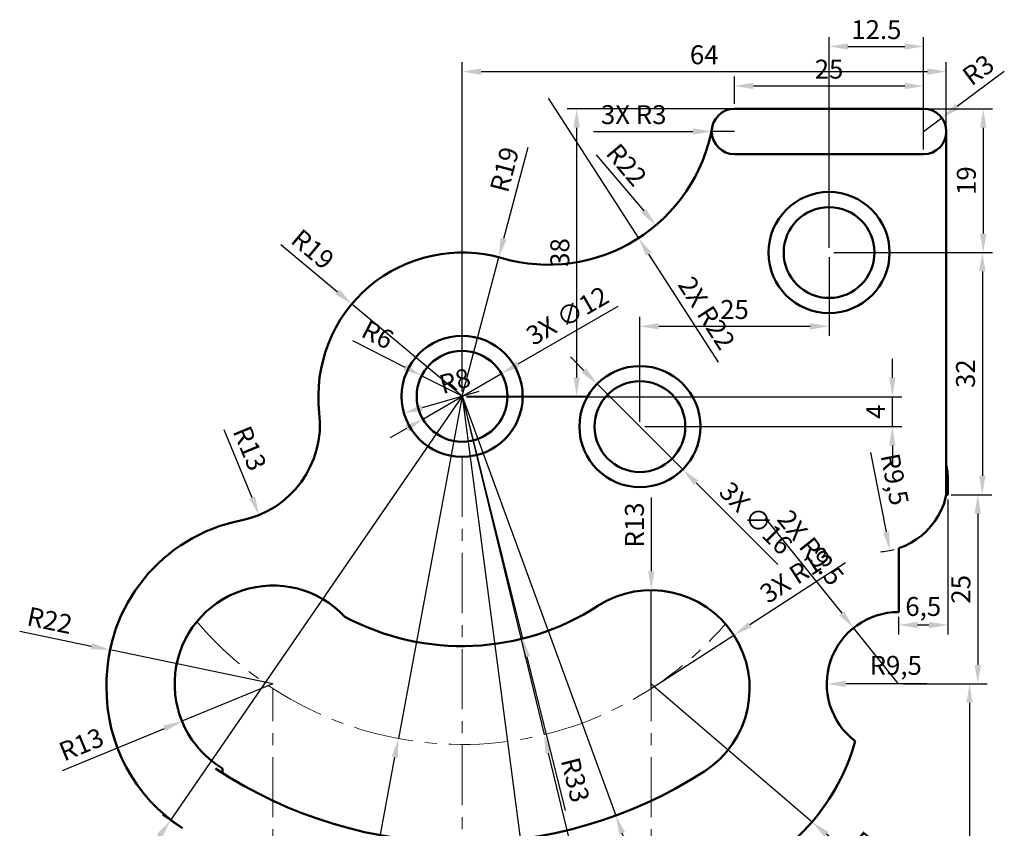
# Model space of a CAD drawing. Units: millimetres. Extents: x 2366 to 2507, y 1526 to 1734.
# Tile 2 of 2: x 2377 to 2507, y 1627 to 1734. Entities that reach past the tile are written whole.
import ezdxf

# ---------------------------------------------------------------- set-up
doc = ezdxf.new("R2010")
doc.units = ezdxf.units.MM
doc.linetypes.add('CENTER', pattern=[50.8, 31.75, -6.35, 6.35, -6.35])
for name, color, linetype, lineweight in [('M-CNTR', 4, 'CENTER', 18), ('M-DIMS', 2, 'Continuous', 25), ('M-OUTL', 7, 'Continuous', 50)]:
    doc.layers.add(name, color=color, linetype=linetype, lineweight=lineweight)
doc.styles.get("Standard").update_dxf_attribs({"font": 'arial.ttf'})
doc.dimstyles.new('ISO-25', dxfattribs={"dimtxt": 2.5, "dimasz": 2.5, "dimexe": 1.25, "dimexo": 0.625, "dimtad": 1, "dimtxsty": 'Standard', "dimcen": 2.5, "dimadec": 0, "dimazin": 0, "dimtfac": 1, "dimtmove": 0, "dimatfit": 3, "dimfxl": 1, "dimarcsym": 0})

# ---------------------------------------------------------------- blocks, each defined once
blk = doc.blocks.new('*D1')
at = {"layer": 'Defpoints', "color": 0, "transparency": 16777216}
for p in [(2496.16, 1724.79), (2471.16, 1721.78), (2496.16, 1721.78)]:
    blk.add_point(p, dxfattribs=at)
at = {"layer": 'M-DIMS', "color": 0, "lineweight": -2, "transparency": 16777216}
for p, q in [((2471.16, 1722.41), (2471.16, 1726.04)), ((2496.16, 1722.41), (2496.16, 1726.04)), ((2473.66, 1724.79), (2493.66, 1724.79))]:
    blk.add_line(p, q, dxfattribs=at)
at = {"layer": 'M-DIMS', "color": 0, "transparency": 16777216}
for points in [[(2473.66, 1725.21), (2473.66, 1724.37), (2471.16, 1724.79)], [(2493.66, 1725.21), (2493.66, 1724.37), (2496.16, 1724.79)]]:
    blk.add_solid(points, dxfattribs=at)
at = {"layer": 'M-DIMS', "color": 0, "transparency": 16777216, "insert": (2483.66, 1726.69), "char_height": 2.5, "attachment_point": 5}
blk.add_mtext('25', dxfattribs=at)
blk = doc.blocks.new('*D2')
at = {"layer": 'Defpoints', "color": 0, "transparency": 16777216}
for p in [(2499.16, 1726.69), (2499.16, 1718.78), (2435.16, 1683.78)]:
    blk.add_point(p, dxfattribs=at)
at = {"layer": 'M-DIMS', "color": 0, "lineweight": -2, "transparency": 16777216}
for p, q in [((2435.16, 1684.41), (2435.16, 1727.94)), ((2499.16, 1719.41), (2499.16, 1727.94)), ((2437.66, 1726.69), (2496.66, 1726.69))]:
    blk.add_line(p, q, dxfattribs=at)
at = {"layer": 'M-DIMS', "color": 0, "transparency": 16777216}
for points in [[(2437.66, 1727.11), (2437.66, 1726.27), (2435.16, 1726.69)], [(2496.66, 1727.11), (2496.66, 1726.27), (2499.16, 1726.69)]]:
    blk.add_solid(points, dxfattribs=at)
at = {"layer": 'M-DIMS', "color": 0, "transparency": 16777216, "insert": (2467.16, 1728.59), "char_height": 2.5, "attachment_point": 5}
blk.add_mtext('64', dxfattribs=at)
blk = doc.blocks.new('*D3')
at = {"layer": 'Defpoints', "color": 0, "transparency": 16777216}
for p in [(2471.16, 1721.78), (2435.16, 1683.78), (2450.3, 1683.78)]:
    blk.add_point(p, dxfattribs=at)
at = {"layer": 'M-DIMS', "color": 0, "lineweight": -2, "transparency": 16777216}
for p, q in [((2470.54, 1721.78), (2449.05, 1721.78)), ((2450.3, 1719.28), (2450.3, 1686.28)), ((2435.79, 1683.78), (2451.55, 1683.78))]:
    blk.add_line(p, q, dxfattribs=at)
at = {"layer": 'M-DIMS', "color": 0, "transparency": 16777216}
for points in [[(2449.89, 1719.28), (2450.72, 1719.28), (2450.3, 1721.78)], [(2449.89, 1686.28), (2450.72, 1686.28), (2450.3, 1683.78)]]:
    blk.add_solid(points, dxfattribs=at)
at = {"layer": 'M-DIMS', "color": 0, "transparency": 16777216, "insert": (2448.4, 1702.78), "char_height": 2.5, "attachment_point": 5, "rotation": 90}
blk.add_mtext('38', dxfattribs=at)
blk = doc.blocks.new('*D4')
at = {"layer": 'Defpoints', "color": 0, "transparency": 16777216}
for p in [(2483.66, 1702.78), (2483.66, 1693.03), (2458.66, 1679.78)]:
    blk.add_point(p, dxfattribs=at)
at = {"layer": 'M-DIMS', "color": 0, "lineweight": -2, "transparency": 16777216}
for p, q in [((2483.66, 1702.16), (2483.66, 1691.78)), ((2458.66, 1680.41), (2458.66, 1694.28)), ((2461.16, 1693.03), (2481.16, 1693.03))]:
    blk.add_line(p, q, dxfattribs=at)
at = {"layer": 'M-DIMS', "color": 0, "transparency": 16777216}
for points in [[(2461.16, 1693.45), (2461.16, 1692.62), (2458.66, 1693.03)], [(2481.16, 1693.45), (2481.16, 1692.62), (2483.66, 1693.03)]]:
    blk.add_solid(points, dxfattribs=at)
at = {"layer": 'M-DIMS', "color": 0, "transparency": 16777216, "insert": (2471.16, 1694.93), "char_height": 2.5, "attachment_point": 5}
blk.add_mtext('25', dxfattribs=at)
blk = doc.blocks.new('*D5')
at = {"layer": 'Defpoints', "color": 0, "transparency": 16777216}
for p in [(2496.16, 1721.78), (2483.66, 1702.78), (2504.03, 1702.78)]:
    blk.add_point(p, dxfattribs=at)
at = {"layer": 'M-DIMS', "color": 0, "lineweight": -2, "transparency": 16777216}
for p, q in [((2496.79, 1721.78), (2505.28, 1721.78)), ((2504.03, 1719.28), (2504.03, 1705.28)), ((2484.29, 1702.78), (2505.28, 1702.78))]:
    blk.add_line(p, q, dxfattribs=at)
at = {"layer": 'M-DIMS', "color": 0, "transparency": 16777216}
for points in [[(2503.62, 1719.28), (2504.45, 1719.28), (2504.03, 1721.78)], [(2503.62, 1705.28), (2504.45, 1705.28), (2504.03, 1702.78)]]:
    blk.add_solid(points, dxfattribs=at)
at = {"layer": 'M-DIMS', "color": 0, "transparency": 16777216, "insert": (2502.13, 1712.28), "char_height": 2.5, "attachment_point": 5, "rotation": 90}
blk.add_mtext('19', dxfattribs=at)
blk = doc.blocks.new('*D6')
at = {"layer": 'Defpoints', "color": 0, "transparency": 16777216}
for p in [(2483.66, 1702.78), (2499.36, 1670.78), (2503.92, 1670.78)]:
    blk.add_point(p, dxfattribs=at)
at = {"layer": 'M-DIMS', "color": 0, "lineweight": -2, "transparency": 16777216}
for p, q in [((2484.29, 1702.78), (2505.17, 1702.78)), ((2503.92, 1700.28), (2503.92, 1673.28)), ((2499.99, 1670.78), (2505.17, 1670.78))]:
    blk.add_line(p, q, dxfattribs=at)
at = {"layer": 'M-DIMS', "color": 0, "transparency": 16777216}
for points in [[(2503.5, 1700.28), (2504.34, 1700.28), (2503.92, 1702.78)], [(2503.5, 1673.28), (2504.34, 1673.28), (2503.92, 1670.78)]]:
    blk.add_solid(points, dxfattribs=at)
at = {"layer": 'M-DIMS', "color": 0, "transparency": 16777216, "insert": (2502.02, 1686.78), "char_height": 2.5, "attachment_point": 5, "rotation": 90}
blk.add_mtext('32', dxfattribs=at)
blk = doc.blocks.new('*D7')
at = {"layer": 'Defpoints', "color": 0, "transparency": 16777216}
for p in [(2499.16, 1670.78), (2492.86, 1645.78), (2503.32, 1645.78)]:
    blk.add_point(p, dxfattribs=at)
at = {"layer": 'M-DIMS', "color": 0, "lineweight": -2, "transparency": 16777216}
for p, q in [((2499.79, 1670.78), (2504.57, 1670.78)), ((2503.32, 1668.28), (2503.32, 1648.28)), ((2493.49, 1645.78), (2504.57, 1645.78))]:
    blk.add_line(p, q, dxfattribs=at)
at = {"layer": 'M-DIMS', "color": 0, "transparency": 16777216}
for points in [[(2502.9, 1668.28), (2503.73, 1668.28), (2503.32, 1670.78)], [(2502.9, 1648.28), (2503.73, 1648.28), (2503.32, 1645.78)]]:
    blk.add_solid(points, dxfattribs=at)
at = {"layer": 'M-DIMS', "color": 0, "transparency": 16777216, "insert": (2501.41, 1658.28), "char_height": 2.5, "attachment_point": 5, "rotation": 90}
blk.add_mtext('25', dxfattribs=at)
blk = doc.blocks.new('*D8')
at = {"layer": 'Defpoints', "color": 0, "transparency": 16777216}
for p in [(2492.86, 1645.78), (2488.16, 1594.78), (2502.23, 1594.78)]:
    blk.add_point(p, dxfattribs=at)
at = {"layer": 'M-DIMS', "color": 0, "lineweight": -2, "transparency": 16777216}
for p, q in [((2493.49, 1645.78), (2503.48, 1645.78)), ((2502.23, 1643.28), (2502.23, 1597.28)), ((2488.79, 1594.78), (2503.48, 1594.78))]:
    blk.add_line(p, q, dxfattribs=at)
at = {"layer": 'M-DIMS', "color": 0, "transparency": 16777216}
for points in [[(2501.81, 1643.28), (2502.64, 1643.28), (2502.23, 1645.78)], [(2501.81, 1597.28), (2502.64, 1597.28), (2502.23, 1594.78)]]:
    blk.add_solid(points, dxfattribs=at)
at = {"layer": 'M-DIMS', "color": 0, "transparency": 16777216, "insert": (2500.33, 1620.28), "char_height": 2.5, "attachment_point": 5, "rotation": 90}
blk.add_mtext('51', dxfattribs=at)
blk = doc.blocks.new('*D9')
at = {"layer": 'Defpoints', "color": 0, "transparency": 16777216}
for p in [(2499.36, 1670.78), (2492.86, 1655.28), (2499.36, 1653.57)]:
    blk.add_point(p, dxfattribs=at)
at = {"layer": 'M-DIMS', "color": 0, "lineweight": -2, "transparency": 16777216}
for p, q in [((2499.36, 1670.16), (2499.36, 1652.32)), ((2492.86, 1654.66), (2492.86, 1652.32)), ((2495.36, 1653.57), (2496.86, 1653.57))]:
    blk.add_line(p, q, dxfattribs=at)
at = {"layer": 'M-DIMS', "color": 0, "transparency": 16777216}
for points in [[(2495.36, 1653.98), (2495.36, 1653.15), (2492.86, 1653.57)], [(2496.86, 1653.98), (2496.86, 1653.15), (2499.36, 1653.57)]]:
    blk.add_solid(points, dxfattribs=at)
at = {"layer": 'M-DIMS', "color": 0, "transparency": 16777216, "insert": (2496.11, 1655.69), "char_height": 2.5, "attachment_point": 5}
blk.add_mtext('6,5', dxfattribs=at)
blk = doc.blocks.new('*D18')
at = {"layer": 'Defpoints', "color": 0, "transparency": 16777216}
for p in [(2435.16, 1683.78), (2426.73, 1638.56)]:
    blk.add_point(p, dxfattribs=at)
at = {"layer": 'M-DIMS', "color": 0, "lineweight": -2, "transparency": 16777216}
for p, q in [((2435.16, 1683.78), (2426.73, 1638.56)), ((2422.8, 1617.49), (2426.27, 1636.1))]:
    blk.add_line(p, q, dxfattribs=at)
at = {"layer": 'M-DIMS', "color": 0, "transparency": 16777216}
blk.add_solid([(2425.86, 1636.18), (2426.68, 1636.03), (2426.73, 1638.56)], dxfattribs=at)
at = {"layer": 'M-DIMS', "color": 0, "transparency": 16777216, "insert": (2421.6, 1621.39), "char_height": 2.5, "attachment_point": 5, "rotation": 79.4409}
blk.add_mtext('R46', dxfattribs=at)
blk = doc.blocks.new('*D19')
at = {"layer": 'Defpoints', "color": 0, "transparency": 16777216}
for p in [(2435.16, 1683.78), (2396.6, 1627.77)]:
    blk.add_point(p, dxfattribs=at)
at = {"layer": 'M-DIMS', "color": 0, "lineweight": -2, "transparency": 16777216}
for p, q in [((2435.16, 1683.78), (2396.6, 1627.77)), ((2389.67, 1617.7), (2395.18, 1625.71))]:
    blk.add_line(p, q, dxfattribs=at)
blk.add_arc((2435.16, 1683.78), 68, 234.401, 236.5526, dxfattribs=at)
at = {"layer": 'M-DIMS', "color": 0, "transparency": 16777216}
blk.add_solid([(2394.84, 1625.95), (2395.53, 1625.48), (2396.6, 1627.77)], dxfattribs=at)
at = {"layer": 'M-DIMS', "color": 0, "transparency": 16777216, "insert": (2390.15, 1621.75), "char_height": 2.5, "attachment_point": 5, "rotation": 55.4543}
blk.add_mtext('R68', dxfattribs=at)
blk = doc.blocks.new('*D20')
at = {"layer": 'Defpoints', "color": 0, "transparency": 16777216}
for p in [(2388.62, 1650.27), (2410.16, 1645.78)]:
    blk.add_point(p, dxfattribs=at)
at = {"layer": 'M-DIMS', "color": 0, "lineweight": -2, "transparency": 16777216}
for p, q in [((2376.68, 1652.75), (2386.18, 1650.78)), ((2410.16, 1645.78), (2388.62, 1650.27))]:
    blk.add_line(p, q, dxfattribs=at)
at = {"layer": 'M-DIMS', "color": 0, "transparency": 16777216}
blk.add_solid([(2386.26, 1651.18), (2386.09, 1650.37), (2388.62, 1650.27)], dxfattribs=at)
at = {"layer": 'M-DIMS', "color": 0, "transparency": 16777216, "insert": (2380.59, 1653.86), "char_height": 2.5, "attachment_point": 5, "rotation": 348.2349}
blk.add_mtext('R22', dxfattribs=at)
blk = doc.blocks.new('*D21')
at = {"layer": 'Defpoints', "color": 0, "transparency": 16777216}
for p in [(2410.16, 1645.78), (2398.13, 1640.85)]:
    blk.add_point(p, dxfattribs=at)
at = {"layer": 'M-DIMS', "color": 0, "lineweight": -2, "transparency": 16777216}
for p, q in [((2410.16, 1645.78), (2398.13, 1640.85)), ((2382.33, 1634.36), (2395.82, 1639.9))]:
    blk.add_line(p, q, dxfattribs=at)
at = {"layer": 'M-DIMS', "color": 0, "transparency": 16777216}
blk.add_solid([(2395.66, 1640.28), (2395.98, 1639.51), (2398.13, 1640.85)], dxfattribs=at)
at = {"layer": 'M-DIMS', "color": 0, "transparency": 16777216, "insert": (2384.95, 1637.49), "char_height": 2.5, "attachment_point": 5, "rotation": 22.313}
blk.add_mtext('R13', dxfattribs=at)
blk = doc.blocks.new('*D22')
at = {"layer": 'Defpoints', "color": 0, "transparency": 16777216}
for p in [(2403.37, 1680.12), (2408.33, 1668.1)]:
    blk.add_point(p, dxfattribs=at)
at = {"layer": 'M-DIMS', "color": 0, "lineweight": -2, "transparency": 16777216}
blk.add_line((2403.67, 1679.4), (2407.38, 1670.41), dxfattribs=at)
at = {"layer": 'M-DIMS', "color": 0, "transparency": 16777216}
blk.add_solid([(2407.77, 1670.57), (2407, 1670.25), (2408.33, 1668.1)], dxfattribs=at)
at = {"layer": 'M-DIMS', "color": 0, "transparency": 16777216, "insert": (2406.81, 1676.79), "char_height": 2.5, "attachment_point": 5, "rotation": 292.4423}
blk.add_mtext('R13', dxfattribs=at)
blk = doc.blocks.new('*D24')
at = {"layer": 'Defpoints', "color": 0, "transparency": 16777216}
for p in [(2460.16, 1645.78), (2481.41, 1627.54)]:
    blk.add_point(p, dxfattribs=at)
at = {"layer": 'M-DIMS', "color": 0, "lineweight": -2, "transparency": 16777216}
for p, q in [((2460.16, 1645.78), (2481.41, 1627.54)), ((2490.69, 1619.58), (2483.3, 1625.92))]:
    blk.add_line(p, q, dxfattribs=at)
at = {"layer": 'M-DIMS', "color": 0, "transparency": 16777216}
blk.add_solid([(2483.58, 1626.23), (2483.03, 1625.6), (2481.41, 1627.54)], dxfattribs=at)
at = {"layer": 'M-DIMS', "color": 0, "transparency": 16777216, "insert": (2489.18, 1623.38), "char_height": 2.5, "attachment_point": 5, "rotation": 319.3585}
blk.add_mtext('R28', dxfattribs=at)
blk = doc.blocks.new('*D25')
at = {"layer": 'Defpoints', "color": 0, "transparency": 16777216}
for p in [(2483.36, 1645.78), (2492.86, 1645.78)]:
    blk.add_point(p, dxfattribs=at)
at = {"layer": 'M-DIMS', "color": 0, "lineweight": -2, "transparency": 16777216}
blk.add_line((2496.58, 1645.78), (2485.86, 1645.78), dxfattribs=at)
at = {"layer": 'M-DIMS', "color": 0, "transparency": 16777216}
blk.add_solid([(2485.86, 1646.2), (2485.86, 1645.36), (2483.36, 1645.78)], dxfattribs=at)
at = {"layer": 'M-DIMS', "color": 0, "transparency": 16777216, "insert": (2492.47, 1647.91), "char_height": 2.5, "attachment_point": 5}
blk.add_mtext('R9,5', dxfattribs=at)
blk = doc.blocks.new('*D26')
at = {"layer": 'Defpoints', "color": 0, "transparency": 16777216}
for p in [(2489.86, 1672.73), (2491.7, 1663.41)]:
    blk.add_point(p, dxfattribs=at)
at = {"layer": 'M-DIMS', "color": 0, "lineweight": -2, "transparency": 16777216}
blk.add_line((2489.15, 1676.37), (2491.21, 1665.86), dxfattribs=at)
blk.add_arc((2489.86, 1672.73), 9.5, 273.5778, 284.639, dxfattribs=at)
at = {"layer": 'M-DIMS', "color": 0, "transparency": 16777216}
blk.add_solid([(2491.62, 1665.94), (2490.8, 1665.78), (2491.7, 1663.41)], dxfattribs=at)
at = {"layer": 'M-DIMS', "color": 0, "transparency": 16777216, "insert": (2492.03, 1672.75), "char_height": 2.5, "attachment_point": 5, "rotation": 281.1167}
blk.add_mtext('R9,5', dxfattribs=at)
blk = doc.blocks.new('*D27')
at = {"layer": 'Defpoints', "color": 0, "transparency": 16777216}
for p in [(2460.16, 1658.17), (2460.16, 1645.17)]:
    blk.add_point(p, dxfattribs=at)
at = {"layer": 'M-DIMS', "color": 0, "lineweight": -2, "transparency": 16777216}
for p, q in [((2460.16, 1670.39), (2460.16, 1660.67)), ((2460.16, 1645.17), (2460.16, 1658.17))]:
    blk.add_line(p, q, dxfattribs=at)
at = {"layer": 'M-DIMS', "color": 0, "transparency": 16777216}
blk.add_solid([(2459.74, 1660.67), (2460.58, 1660.67), (2460.16, 1658.17)], dxfattribs=at)
at = {"layer": 'M-DIMS', "color": 0, "transparency": 16777216, "insert": (2458.26, 1666.78), "char_height": 2.5, "attachment_point": 5, "rotation": 90}
blk.add_mtext('R13', dxfattribs=at)
blk = doc.blocks.new('*D28')
at = {"layer": 'Defpoints', "color": 0, "transparency": 16777216}
for p in [(2435.16, 1683.78), (2427.47, 1681.57)]:
    blk.add_point(p, dxfattribs=at)
at = {"layer": 'M-DIMS', "color": 0, "lineweight": -2, "transparency": 16777216}
blk.add_line((2437.36, 1684.41), (2429.88, 1682.26), dxfattribs=at)
at = {"layer": 'M-DIMS', "color": 0, "transparency": 16777216}
blk.add_solid([(2429.76, 1682.66), (2429.99, 1681.86), (2427.47, 1681.57)], dxfattribs=at)
at = {"layer": 'M-DIMS', "color": 0, "transparency": 16777216, "insert": (2434.29, 1685.51), "char_height": 2.5, "attachment_point": 5, "rotation": 16.0232}
blk.add_mtext('R8', dxfattribs=at)
blk = doc.blocks.new('*D29')
at = {"layer": 'Defpoints', "color": 0, "transparency": 16777216}
for p in [(2429.81, 1686.5), (2435.16, 1683.78)]:
    blk.add_point(p, dxfattribs=at)
at = {"layer": 'M-DIMS', "color": 0, "lineweight": -2, "transparency": 16777216}
for p, q in [((2420.65, 1691.15), (2427.58, 1687.63)), ((2435.16, 1683.78), (2429.81, 1686.5))]:
    blk.add_line(p, q, dxfattribs=at)
at = {"layer": 'M-DIMS', "color": 0, "transparency": 16777216}
blk.add_solid([(2427.77, 1688), (2427.39, 1687.26), (2429.81, 1686.5)], dxfattribs=at)
at = {"layer": 'M-DIMS', "color": 0, "transparency": 16777216, "insert": (2423.86, 1691.65), "char_height": 2.5, "attachment_point": 5, "rotation": 333.0794}
blk.add_mtext('R6', dxfattribs=at)
blk = doc.blocks.new('*D30')
at = {"layer": 'Defpoints', "color": 0, "transparency": 16777216}
for p in [(2420.6, 1695.98), (2435.16, 1683.78)]:
    blk.add_point(p, dxfattribs=at)
at = {"layer": 'M-DIMS', "color": 0, "lineweight": -2, "transparency": 16777216}
for p, q in [((2411.22, 1703.84), (2418.68, 1697.59)), ((2435.16, 1683.78), (2420.6, 1695.98))]:
    blk.add_line(p, q, dxfattribs=at)
at = {"layer": 'M-DIMS', "color": 0, "transparency": 16777216}
blk.add_solid([(2418.95, 1697.91), (2418.41, 1697.27), (2420.6, 1695.98)], dxfattribs=at)
at = {"layer": 'M-DIMS', "color": 0, "transparency": 16777216, "insert": (2415.21, 1702.97), "char_height": 2.5, "attachment_point": 5, "rotation": 320.0449}
blk.add_mtext('R19', dxfattribs=at)
blk = doc.blocks.new('*D31')
at = {"layer": 'Defpoints', "color": 0, "transparency": 16777216}
for p in [(2446.55, 1723.17), (2460.77, 1706.38)]:
    blk.add_point(p, dxfattribs=at)
at = {"layer": 'M-DIMS', "color": 0, "lineweight": -2, "transparency": 16777216}
blk.add_line((2452.89, 1715.69), (2459.16, 1708.29), dxfattribs=at)
at = {"layer": 'M-DIMS', "color": 0, "transparency": 16777216}
blk.add_solid([(2459.47, 1708.56), (2458.84, 1708.02), (2460.77, 1706.38)], dxfattribs=at)
at = {"layer": 'M-DIMS', "color": 0, "transparency": 16777216, "insert": (2456.65, 1714.16), "char_height": 2.5, "attachment_point": 5, "rotation": 310.2815}
blk.add_mtext('R22', dxfattribs=at)
blk = doc.blocks.new('*D32')
at = {"layer": 'Defpoints', "color": 0, "transparency": 16777216}
for p in [(2498.57, 1720.57), (2496.16, 1718.78)]:
    blk.add_point(p, dxfattribs=at)
at = {"layer": 'M-DIMS', "color": 0, "lineweight": -2, "transparency": 16777216}
for p, q in [((2506.82, 1726.7), (2500.58, 1722.06)), ((2496.16, 1718.78), (2498.57, 1720.57))]:
    blk.add_line(p, q, dxfattribs=at)
at = {"layer": 'M-DIMS', "color": 0, "transparency": 16777216}
blk.add_solid([(2500.33, 1722.39), (2500.83, 1721.73), (2498.57, 1720.57)], dxfattribs=at)
at = {"layer": 'M-DIMS', "color": 0, "transparency": 16777216, "insert": (2503.57, 1726.65), "char_height": 2.5, "attachment_point": 5, "rotation": 36.6003}
blk.add_mtext('R3', dxfattribs=at)
blk = doc.blocks.new('*D33')
at = {"layer": 'Defpoints', "color": 0, "transparency": 16777216}
for p in [(2435.12, 1683.73), (2492.03, 1683.73), (2458.66, 1679.78)]:
    blk.add_point(p, dxfattribs=at)
at = {"layer": 'M-DIMS', "color": 0, "lineweight": -2, "transparency": 16777216}
for p, q in [((2492.03, 1686.23), (2492.03, 1688.73)), ((2435.75, 1683.73), (2493.28, 1683.73)), ((2492.03, 1679.78), (2492.03, 1683.73)), ((2459.29, 1679.78), (2493.28, 1679.78)), ((2492.03, 1677.28), (2492.03, 1674.78))]:
    blk.add_line(p, q, dxfattribs=at)
at = {"layer": 'M-DIMS', "color": 0, "transparency": 16777216}
for points in [[(2491.61, 1686.23), (2492.44, 1686.23), (2492.03, 1683.73)], [(2491.61, 1677.28), (2492.44, 1677.28), (2492.03, 1679.78)]]:
    blk.add_solid(points, dxfattribs=at)
at = {"layer": 'M-DIMS', "color": 0, "transparency": 16777216, "insert": (2490.15, 1681.75), "char_height": 2.5, "attachment_point": 5, "rotation": 90}
blk.add_mtext('4', dxfattribs=at)
blk = doc.blocks.new('MOUNT-HOLE-D12-D16')
for radius in [8, 6]:
    blk.add_circle((0, 0), radius)
blk = doc.blocks.new('*D35')
at = {"layer": 'Defpoints', "color": 0, "transparency": 16777216}
for p in [(2496.16, 1730.01), (2496.16, 1715.78), (2483.66, 1702.78)]:
    blk.add_point(p, dxfattribs=at)
at = {"layer": 'M-DIMS', "color": 0, "lineweight": -2, "transparency": 16777216}
for p, q in [((2483.66, 1703.41), (2483.66, 1731.26)), ((2496.16, 1716.41), (2496.16, 1731.26)), ((2486.16, 1730.01), (2493.66, 1730.01))]:
    blk.add_line(p, q, dxfattribs=at)
at = {"layer": 'M-DIMS', "color": 0, "transparency": 16777216}
for points in [[(2486.16, 1730.42), (2486.16, 1729.59), (2483.66, 1730.01)], [(2493.66, 1730.42), (2493.66, 1729.59), (2496.16, 1730.01)]]:
    blk.add_solid(points, dxfattribs=at)
at = {"layer": 'M-DIMS', "color": 0, "transparency": 16777216, "insert": (2489.91, 1731.91), "char_height": 2.5, "attachment_point": 5}
blk.add_mtext('12.5', dxfattribs=at)
blk = doc.blocks.new('*D36')
at = {"layer": 'Defpoints', "color": 0, "transparency": 16777216}
for p in [(2440.36, 1686.78), (2429.96, 1680.78)]:
    blk.add_point(p, dxfattribs=at)
at = {"layer": 'M-DIMS', "color": 0, "lineweight": -2, "transparency": 16777216}
for p, q in [((2455.74, 1695.65), (2442.52, 1688.03)), ((2429.96, 1680.78), (2440.36, 1686.78)), ((2427.8, 1679.53), (2425.63, 1678.28))]:
    blk.add_line(p, q, dxfattribs=at)
at = {"layer": 'M-DIMS', "color": 0, "transparency": 16777216}
for points in [[(2442.32, 1688.39), (2442.73, 1687.67), (2440.36, 1686.78)], [(2427.59, 1679.89), (2428.01, 1679.17), (2429.96, 1680.78)]]:
    blk.add_solid(points, dxfattribs=at)
at = {"layer": 'M-DIMS', "color": 0, "transparency": 16777216, "insert": (2449.23, 1694.17), "char_height": 2.5, "attachment_point": 5, "rotation": 29.9793}
blk.add_mtext('3X ∅12', dxfattribs=at)
blk = doc.blocks.new('*D37')
at = {"layer": 'Defpoints', "color": 0, "transparency": 16777216}
for p in [(2453.01, 1685.44), (2464.32, 1674.12)]:
    blk.add_point(p, dxfattribs=at)
at = {"layer": 'M-DIMS', "color": 0, "lineweight": -2, "transparency": 16777216}
for p, q in [((2451.24, 1687.21), (2449.47, 1688.98)), ((2453.01, 1685.44), (2464.32, 1674.12)), ((2476.89, 1661.54), (2466.08, 1672.35))]:
    blk.add_line(p, q, dxfattribs=at)
at = {"layer": 'M-DIMS', "color": 0, "transparency": 16777216}
for points in [[(2451.53, 1687.5), (2450.94, 1686.91), (2453.01, 1685.44)], [(2466.38, 1672.65), (2465.79, 1672.06), (2464.32, 1674.12)]]:
    blk.add_solid(points, dxfattribs=at)
at = {"layer": 'M-DIMS', "color": 0, "transparency": 16777216, "insert": (2473.77, 1667.46), "char_height": 2.5, "attachment_point": 5, "rotation": 314.9877}
blk.add_mtext('3X ∅16', dxfattribs=at)
blk = doc.blocks.new('*D38')
at = {"layer": 'Defpoints', "color": 0, "transparency": 16777216}
for p in [(2435.16, 1683.78), (2447.8, 1587.61)]:
    blk.add_point(p, dxfattribs=at)
at = {"layer": 'M-DIMS', "color": 0, "lineweight": -2, "transparency": 16777216}
for p, q in [((2435.16, 1683.78), (2447.8, 1587.61)), ((2455.85, 1526.32), (2448.13, 1585.13))]:
    blk.add_line(p, q, dxfattribs=at)
at = {"layer": 'M-DIMS', "color": 0, "transparency": 16777216}
blk.add_solid([(2448.54, 1585.18), (2447.71, 1585.08), (2447.8, 1587.61)], dxfattribs=at)
at = {"layer": 'M-DIMS', "color": 0, "transparency": 16777216, "insert": (2457.27, 1530.15), "char_height": 2.5, "attachment_point": 5, "rotation": 277.4868}
blk.add_mtext('R97', dxfattribs=at)
blk = doc.blocks.new('*D39')
at = {"layer": 'Defpoints', "color": 0, "transparency": 16777216}
for p in [(2435.16, 1683.78), (2455.46, 1628.38)]:
    blk.add_point(p, dxfattribs=at)
at = {"layer": 'M-DIMS', "color": 0, "lineweight": -2, "transparency": 16777216}
for p, q in [((2435.16, 1683.78), (2455.46, 1628.38)), ((2468.89, 1591.75), (2456.32, 1626.04))]:
    blk.add_line(p, q, dxfattribs=at)
at = {"layer": 'M-DIMS', "color": 0, "transparency": 16777216}
blk.add_solid([(2456.71, 1626.18), (2455.93, 1625.89), (2455.46, 1628.38)], dxfattribs=at)
at = {"layer": 'M-DIMS', "color": 0, "transparency": 16777216, "insert": (2469.43, 1595.8), "char_height": 2.5, "attachment_point": 5, "rotation": 290.1259}
blk.add_mtext('R59', dxfattribs=at)
blk = doc.blocks.new('*D40')
at = {"layer": 'Defpoints', "color": 0, "transparency": 16777216}
for p in [(2435.16, 1683.78), (2446, 1639.08)]:
    blk.add_point(p, dxfattribs=at)
at = {"layer": 'M-DIMS', "color": 0, "lineweight": -2, "transparency": 16777216}
for p, q in [((2435.16, 1683.78), (2446, 1639.08)), ((2453.36, 1608.74), (2446.59, 1636.65))]:
    blk.add_line(p, q, dxfattribs=at)
at = {"layer": 'M-DIMS', "color": 0, "transparency": 16777216}
blk.add_solid([(2446.99, 1636.75), (2446.19, 1636.55), (2446, 1639.08)], dxfattribs=at)
at = {"layer": 'M-DIMS', "color": 0, "transparency": 16777216, "insert": (2454.35, 1612.7), "char_height": 2.5, "attachment_point": 5, "rotation": 283.6294}
blk.add_mtext('R46', dxfattribs=at)
blk = doc.blocks.new('*D41')
at = {"layer": 'Defpoints', "color": 0, "transparency": 16777216}
for p in [(2435.16, 1683.78), (2443.16, 1651.77)]:
    blk.add_point(p, dxfattribs=at)
at = {"layer": 'M-DIMS', "color": 0, "lineweight": -2, "transparency": 16777216}
for p, q in [((2435.16, 1683.78), (2443.16, 1651.77)), ((2448.84, 1629.05), (2443.77, 1649.34))]:
    blk.add_line(p, q, dxfattribs=at)
at = {"layer": 'M-DIMS', "color": 0, "transparency": 16777216}
blk.add_solid([(2444.17, 1649.44), (2443.36, 1649.24), (2443.16, 1651.77)], dxfattribs=at)
at = {"layer": 'M-DIMS', "color": 0, "transparency": 16777216, "insert": (2449.81, 1633.02), "char_height": 2.5, "attachment_point": 5, "rotation": 284.0293}
blk.add_mtext('R33', dxfattribs=at)
blk = doc.blocks.new('*D43')
at = {"layer": 'Defpoints', "color": 0, "transparency": 16777216}
for p in [(2446.55, 1723.17), (2458.48, 1704.68)]:
    blk.add_point(p, dxfattribs=at)
at = {"layer": 'M-DIMS', "color": 0, "lineweight": -2, "transparency": 16777216}
for p, q in [((2446.55, 1723.17), (2458.48, 1704.68)), ((2469.06, 1688.29), (2459.83, 1702.58))]:
    blk.add_line(p, q, dxfattribs=at)
at = {"layer": 'M-DIMS', "color": 0, "transparency": 16777216}
blk.add_solid([(2460.18, 1702.81), (2459.48, 1702.36), (2458.48, 1704.68)], dxfattribs=at)
at = {"layer": 'M-DIMS', "color": 0, "transparency": 16777216, "insert": (2467.22, 1694.61), "char_height": 2.5, "attachment_point": 5, "rotation": 302.8368}
blk.add_mtext('2X R22', dxfattribs=at)
blk = doc.blocks.new('*D44')
at = {"layer": 'Defpoints', "color": 0, "transparency": 16777216}
for p in [(2440, 1702.15), (2435.16, 1683.78)]:
    blk.add_point(p, dxfattribs=at)
at = {"layer": 'M-DIMS', "color": 0, "lineweight": -2, "transparency": 16777216}
for p, q in [((2443.83, 1716.67), (2440.64, 1704.57)), ((2435.16, 1683.78), (2440, 1702.15))]:
    blk.add_line(p, q, dxfattribs=at)
at = {"layer": 'M-DIMS', "color": 0, "transparency": 16777216}
blk.add_solid([(2440.24, 1704.68), (2441.04, 1704.47), (2440, 1702.15)], dxfattribs=at)
at = {"layer": 'M-DIMS', "color": 0, "transparency": 16777216, "insert": (2441.07, 1713.66), "char_height": 2.5, "attachment_point": 5, "rotation": 75.2427}
blk.add_mtext('R19', dxfattribs=at)
blk = doc.blocks.new('*D45')
at = {"layer": 'Defpoints', "color": 0, "transparency": 16777216}
for p in [(2471.07, 1652.23), (2460.16, 1645.17)]:
    blk.add_point(p, dxfattribs=at)
at = {"layer": 'M-DIMS', "color": 0, "lineweight": -2, "transparency": 16777216}
for p, q in [((2485.84, 1661.79), (2473.17, 1653.59)), ((2460.16, 1645.17), (2471.07, 1652.23))]:
    blk.add_line(p, q, dxfattribs=at)
at = {"layer": 'M-DIMS', "color": 0, "transparency": 16777216}
blk.add_solid([(2472.95, 1653.94), (2473.4, 1653.24), (2471.07, 1652.23)], dxfattribs=at)
at = {"layer": 'M-DIMS', "color": 0, "transparency": 16777216, "insert": (2479.52, 1659.97), "char_height": 2.5, "attachment_point": 5, "rotation": 32.9211}
blk.add_mtext('3X R13', dxfattribs=at)
blk = doc.blocks.new('*D46')
at = {"layer": 'Defpoints', "color": 0, "transparency": 16777216}
for p in [(2486.91, 1653.18), (2492.86, 1645.78)]:
    blk.add_point(p, dxfattribs=at)
at = {"layer": 'M-DIMS', "color": 0, "lineweight": -2, "transparency": 16777216}
for p, q in [((2475.23, 1667.69), (2485.34, 1655.13)), ((2492.86, 1645.78), (2486.91, 1653.18))]:
    blk.add_line(p, q, dxfattribs=at)
at = {"layer": 'M-DIMS', "color": 0, "transparency": 16777216}
blk.add_solid([(2485.66, 1655.39), (2485.01, 1654.87), (2486.91, 1653.18)], dxfattribs=at)
at = {"layer": 'M-DIMS', "color": 0, "transparency": 16777216, "insert": (2480.98, 1663.58), "char_height": 2.5, "attachment_point": 5, "rotation": 308.8308}
blk.add_mtext('2X R9.5', dxfattribs=at)
blk = doc.blocks.new('*D48')
at = {"layer": 'Defpoints', "color": 0, "transparency": 16777216}
for p in [(2468.16, 1718.78), (2471.16, 1718.78)]:
    blk.add_point(p, dxfattribs=at)
at = {"layer": 'M-DIMS', "color": 0, "lineweight": -2, "transparency": 16777216}
for p, q in [((2452.51, 1718.78), (2465.66, 1718.78)), ((2471.16, 1718.78), (2468.16, 1718.78))]:
    blk.add_line(p, q, dxfattribs=at)
at = {"layer": 'M-DIMS', "color": 0, "transparency": 16777216}
blk.add_solid([(2465.66, 1719.2), (2465.66, 1718.36), (2468.16, 1718.78)], dxfattribs=at)
at = {"layer": 'M-DIMS', "color": 0, "transparency": 16777216, "insert": (2457.84, 1720.68), "char_height": 2.5, "attachment_point": 5, "rotation": 0.0013}
blk.add_mtext('3X R3', dxfattribs=at)

msp = doc.modelspace()

# ---------------------------------------------------------------- linework, layer by layer
at = {"layer": 'M-CNTR', "ltscale": 0.25}
for p, q in [((2435.161, 1675.781), (2435.161, 1626.165)), ((2410.161, 1590.058), (2410.161, 1645.168)), ((2460.161, 1590.058), (2460.161, 1645.168))]:
    msp.add_line(p, q, dxfattribs=at)
msp.add_arc((2435.161, 1683.781), 46, 220.33337, 319.1674, dxfattribs=at)
at = {"layer": 'M-OUTL'}
for p, q in [((2496.161, 1721.781), (2471.161, 1721.781)), ((2499.161, 1718.781), (2499.161, 1702.781)), ((2496.161, 1715.781), (2471.161, 1715.781)), ((2499.161, 1702.781), (2499.161, 1670.781)), ((2499.363, 1672.73), (2499.363, 1670.781)), ((2499.363, 1670.781), (2499.161, 1670.781)), ((2492.863, 1663.716), (2492.863, 1655.281)), ((2403.474, 1634.012), (2403.497, 1634.619))]:
    msp.add_line(p, q, dxfattribs=at)
for centre, radius, start, end in [((2471.161, 1718.781), 3, 90, 270), ((2496.161, 1718.781), 3, 270, 90), ((2446.549, 1723.168), 22, 253.87385, 349.89399), ((2435.161, 1683.781), 19, 73.87385, 186.5763), ((2403.372, 1680.116), 13, 281.18539, 6.5763), ((2489.863, 1672.73), 9.5, 288.40848, 11.83993), ((2410.161, 1645.781), 22, 101.14047, 180.79887), ((2410.161, 1645.781), 13, 42.9602, 239.16153), ((2460.161, 1645.168), 13, 302.92073, 122.92073), ((2435.161, 1683.781), 33, 242.01242, 302.92073), ((2492.863, 1645.781), 9.5, 90, 232.79807), ((2410.161, 1645.168), 22, 179.20113, 237.07927), ((2460.161, 1645.781), 28, 294.39575, 344.32119), ((2435.161, 1683.781), 59, 236.4813, 302.92073)]:
    msp.add_arc(centre, radius, start, end, dxfattribs=at)

# ---------------------------------------------------------------- block references
for p in [(2483.661, 1702.781), (2435.161, 1683.781), (2458.661, 1679.781)]:
    msp.add_blockref('MOUNT-HOLE-D12-D16', p, dxfattribs=at)

# ---------------------------------------------------------------- dimensions: what is measured, and where the dimension line sits
at = {"layer": 'M-DIMS'}
for base, p1, p2, override, picture, middle in [((2496.161, 1730.006), (2483.661, 1702.781), (2496.161, 1715.781), {"dimdec": 1, "dimlfac": 1, "dimrnd": 0, "dimzin": 0, "dimdsep": 46, "dimlunit": 2}, '*D35', (2489.911, 1731.908)), ((2499.161, 1726.69), (2435.161, 1683.781), (2499.161, 1718.781), {"dimclrd": 0, "dimclre": 0, "dimclrt": 0}, '*D2', (2467.161, 1728.591)), ((2496.161, 1724.789), (2471.161, 1721.781), (2496.161, 1721.781), {"dimclrd": 0, "dimclre": 0, "dimclrt": 0}, '*D1', (2483.661, 1726.69)), ((2483.661, 1693.032), (2458.661, 1679.781), (2483.661, 1702.781), {"dimclrd": 0, "dimclre": 0, "dimclrt": 0}, '*D4', (2471.161, 1694.933)), ((2499.363, 1653.566), (2492.863, 1655.281), (2499.363, 1670.781), {"dimclrd": 0, "dimclre": 0, "dimclrt": 0}, '*D9', (2496.113, 1655.693))]:
    dim = msp.add_linear_dim(base=base, p1=p1, p2=p2, dimstyle='ISO-25', override=override, dxfattribs=at)
    dim.commit()
    dim.dimension.update_dxf_attribs({"geometry": picture, "text_midpoint": middle})
for center, mpoint, picture, middle in [((2496.161, 1718.781), (2498.57, 1720.57), '*D32', (2503.57, 1726.653)), ((2435.161, 1683.781), (2420.597, 1695.983), '*D30', (2415.215, 1702.972)), ((2435.161, 1683.781), (2429.812, 1686.498), '*D29', (2423.861, 1691.652)), ((2435.161, 1683.781), (2396.601, 1627.771), '*D19', (2390.15, 1621.754)), ((2460.161, 1645.168), (2460.161, 1658.168), '*D27', (2458.259, 1666.779)), ((2410.161, 1645.781), (2388.624, 1650.267), '*D20', (2380.588, 1653.861)), ((2460.161, 1645.781), (2481.408, 1627.544), '*D24', (2489.183, 1623.376))]:
    dim = msp.add_radius_dim(center=center, mpoint=mpoint, dimstyle='ISO-25', override={"dimclrd": 0, "dimclre": 0, "dimclrt": 0}, dxfattribs=at)
    dim.commit()
    dim.dimension.update_dxf_attribs({"geometry": picture, "text_midpoint": middle})
for center, mpoint, text, override, picture, middle in [((2471.161, 1718.781), (2468.161, 1718.781), '3X <>', {"dimdec": 0, "dimlfac": 1, "dimrnd": 0, "dimzin": 0, "dimdsep": 46, "dimlunit": 2}, '*D48', (2457.836, 1720.683)), ((2492.863, 1645.781), (2486.907, 1653.182), '2X <>', {"dimdec": 1, "dimlfac": 1, "dimrnd": 0, "dimzin": 0, "dimdsep": 46, "dimlunit": 2}, '*D46', (2480.981, 1663.577)), ((2460.161, 1645.168), (2471.074, 1652.233), '3X <>', {"dimdec": 0, "dimlfac": 1, "dimrnd": 0, "dimzin": 0, "dimdsep": 46, "dimlunit": 2}, '*D45', (2479.523, 1659.969))]:
    dim = msp.add_radius_dim(center=center, mpoint=mpoint, text=text, dimstyle='ISO-25', override=override, dxfattribs=at)
    dim.commit()
    dim.dimension.update_dxf_attribs({"geometry": picture, "text_midpoint": middle})
for center, mpoint, override, picture, middle in [((2446.549, 1723.168), (2460.773, 1706.385), {"dimclrd": 0, "dimclre": 0, "dimclrt": 0}, '*D31', (2455.214, 1712.945)), ((2435.161, 1683.781), (2440.001, 1702.154), {"dimdec": 0, "dimlfac": 1, "dimrnd": 0, "dimzin": 0, "dimdsep": 46, "dimlunit": 2}, '*D44', (2442.905, 1713.178)), ((2435.161, 1683.781), (2427.472, 1681.573), {"dimclrd": 0, "dimclre": 0, "dimclrt": 0}, '*D28', (2434.818, 1683.683)), ((2435.161, 1683.781), (2426.732, 1638.56), {"dimclrd": 0, "dimclre": 0, "dimclrt": 0}, '*D18', (2423.466, 1621.04)), ((2435.161, 1683.781), (2447.8, 1587.608), {"dimdec": 0, "dimlfac": 1, "dimrnd": 0, "dimzin": 0, "dimdsep": 46, "dimlunit": 2}, '*D38', (2455.384, 1529.904)), ((2435.161, 1683.781), (2455.462, 1628.384), {"dimdec": 0, "dimlfac": 1, "dimrnd": 0, "dimzin": 0, "dimdsep": 46, "dimlunit": 2}, '*D39', (2467.643, 1595.145)), ((2435.161, 1683.781), (2446.001, 1639.076), {"dimdec": 0, "dimlfac": 1, "dimrnd": 0, "dimzin": 0, "dimdsep": 46, "dimlunit": 2}, '*D40', (2452.505, 1612.254)), ((2435.161, 1683.781), (2443.161, 1651.765), {"dimdec": 0, "dimlfac": 1, "dimrnd": 0, "dimzin": 0, "dimdsep": 46, "dimlunit": 2}, '*D41', (2447.961, 1632.556)), ((2403.372, 1680.116), (2408.335, 1668.101), {"dimclrd": 0, "dimclre": 0, "dimclrt": 0}, '*D22', (2405.047, 1676.06)), ((2489.863, 1672.73), (2491.695, 1663.409), {"dimclrd": 0, "dimclre": 0, "dimclrt": 0}, '*D26', (2489.939, 1672.344)), ((2492.863, 1645.781), (2483.363, 1645.781), {"dimclrd": 0, "dimclre": 0, "dimclrt": 0}, '*D25', (2492.47, 1645.781)), ((2410.161, 1645.781), (2398.135, 1640.845), {"dimclrd": 0, "dimclre": 0, "dimclrt": 0}, '*D21', (2385.668, 1635.729))]:
    dim = msp.add_radius_dim(center=center, mpoint=mpoint, dimstyle='ISO-25', override=override, dxfattribs=at)
    dim.commit()
    dim.dimension.update_dxf_attribs({"geometry": picture, "text_midpoint": middle, "dimtype": 164})
dim = msp.add_radius_dim(center=(2446.549, 1723.168), mpoint=(2458.479, 1704.683), text='2X <>', dimstyle='ISO-25', override={"dimdec": 0, "dimlfac": 1, "dimrnd": 0, "dimzin": 0, "dimdsep": 46, "dimlunit": 2}, dxfattribs=at)
dim.commit()
dim.dimension.update_dxf_attribs({"geometry": '*D43', "text_midpoint": (2465.636, 1693.592), "dimtype": 164})
for base, p1, p2, override, picture, middle in [((2450.302, 1683.781), (2471.161, 1721.781), (2435.161, 1683.781), {"dimclrd": 0, "dimclre": 0, "dimclrt": 0}, '*D3', (2448.4, 1702.781)), ((2504.035, 1702.781), (2496.161, 1721.781), (2483.661, 1702.781), {"dimclrd": 0, "dimclre": 0, "dimclrt": 0}, '*D5', (2502.133, 1712.281)), ((2503.919, 1670.781), (2483.661, 1702.781), (2499.363, 1670.781), {"dimclrd": 0, "dimclre": 0, "dimclrt": 0}, '*D6', (2502.017, 1686.781)), ((2492.027, 1683.726), (2458.661, 1679.781), (2435.124, 1683.726), {"dimdec": 0, "dimclrd": 0, "dimclre": 0, "dimclrt": 0}, '*D33', (2490.152, 1681.754)), ((2503.316, 1645.781), (2499.161, 1670.781), (2492.863, 1645.781), {"dimclrd": 0, "dimclre": 0, "dimclrt": 0}, '*D7', (2501.415, 1658.281)), ((2502.227, 1594.781), (2492.863, 1645.781), (2488.161, 1594.781), {"dimclrd": 0, "dimclre": 0, "dimclrt": 0}, '*D8', (2500.325, 1620.281))]:
    dim = msp.add_linear_dim(base=base, p1=p1, p2=p2, angle=90, dimstyle='ISO-25', override=override, dxfattribs=at)
    dim.commit()
    dim.dimension.update_dxf_attribs({"geometry": picture, "text_midpoint": middle})
dim = msp.add_diameter_dim_2p(p1=(2429.964, 1680.783), p2=(2440.359, 1686.779), text='3X <>', dimstyle='ISO-25', override={"dimdec": 0, "dimlfac": 1, "dimrnd": 0, "dimzin": 0, "dimdsep": 46, "dimlunit": 2}, dxfattribs=at)
dim.commit()
dim.dimension.update_dxf_attribs({"geometry": '*D36', "text_midpoint": (2450.217, 1692.466), "dimtype": 163})
dim = msp.add_diameter_dim_2p(p1=(2453.006, 1685.439), p2=(2464.317, 1674.123), text='3X <>', dimstyle='ISO-25', override={"dimdec": 0, "dimlfac": 1, "dimrnd": 0, "dimzin": 0, "dimdsep": 46, "dimlunit": 2}, dxfattribs=at)
dim.commit()
dim.dimension.update_dxf_attribs({"geometry": '*D37', "text_midpoint": (2472.372, 1666.065)})

doc.saveas('drawing.dxf')
